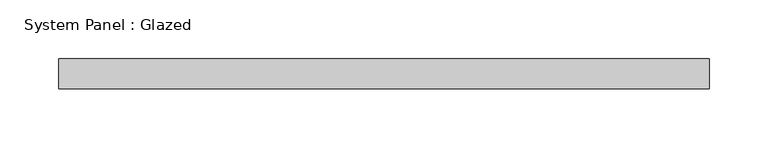
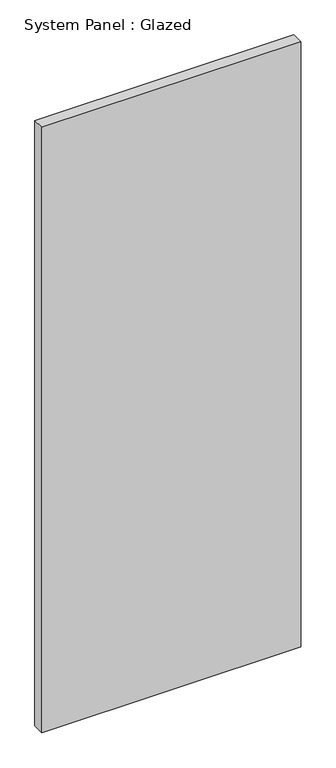
"""IFC4 building model written with IfcOpenShell, lengths in millimetres: plate geometry, System Panel : Glazed."""

from ifc_helpers import new_model, si_unit, origin, origin_with_axes, place, context, project, spatial, polyline, outline, extrude, source, transform, mapped, element, save


def system_panel_glazed_6dadbfa4(model_context):
    return source(origin(), model_context, "Body", "SweptSolid", [
        extrude(outline(polyline([(276.225, 19.05), (-276.225, 19.05), (-276.225, 44.45), (276.225, 44.45), (276.225, 19.05)])), origin_with_axes(), (0.0, 0.0, 1.0), 1366.5474484),
    ])


if __name__ == "__main__":
    model = new_model("IFC4")
    model_context = context("Model", 3, world=origin())
    ifc_project = project(units=[si_unit("LENGTHUNIT", "METRE", prefix="MILLI")], contexts=[model_context])
    site = spatial("IfcSite", under=ifc_project)
    building = spatial("IfcBuilding", under=site)
    placement = place(None, origin())
    system_panel_glazed_shape = system_panel_glazed_6dadbfa4(model_context)
    element("IfcPlate", 1, ObjectType="System Panel : Glazed", at=placement, inside=building, context=model_context, shape_type="MappedRepresentation", body=[
        mapped(system_panel_glazed_shape, transform((0.0, 0.0, 0.0), x_axis=(1.0, 0.0, 0.0), y_axis=(0.0, 1.0, 0.0), z_axis=(0.0, 0.0, 1.0))),
    ])
    save(model, "model.ifc")

# Revit data of these elements
# Type "System Panel : Glazed"
#   Construction Type Id = "GSP4R"
#   Analytic Construction = "1/8 in Pilkington single glazing"
#   Visual Light Transmittance = 0.9
#   Solar Heat Gain Coefficient = 0.86
#   Heat Transfer Coefficient (U) = 1.18115 BTU/(h·ft²·°F)
#   Define Thermal Properties by = 1
# Element 1 (IfcPlate, "System Panel : Glazed")
#   Materials on its faces: "Glass"
# Materials
#   "Glass": class "Glass", colour RGB 0 128 192, transparency 0.75, Description = "Soda Lime Glass", Cost = 0
